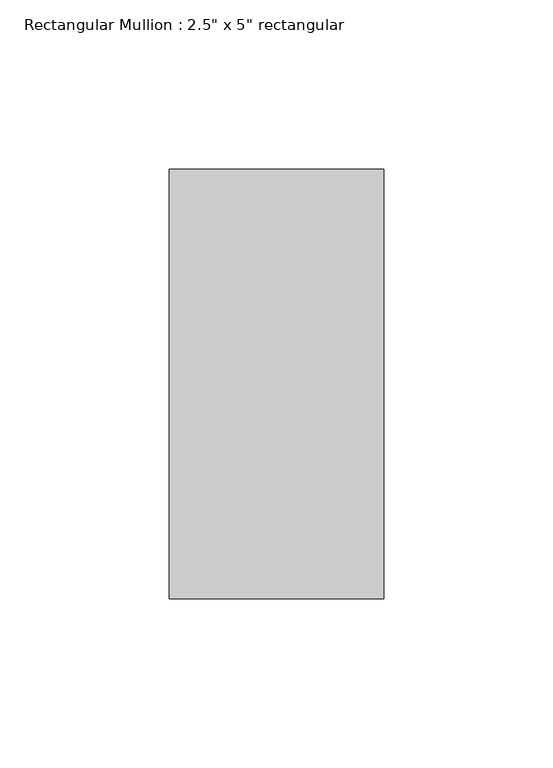
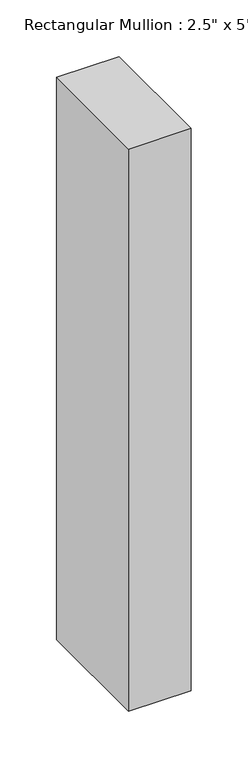
"""IFC4 building model written with IfcOpenShell, lengths in millimetres: member geometry."""

from ifc_helpers import new_model, si_unit, frame, origin, place, context, project, spatial, polyline, outline, extrude, source, transform, mapped, element, save


def member_00d8fd3b(model_context):
    return source(origin(), model_context, "Body", "SweptSolid", [
        extrude(outline(polyline([(0.0, 63.5), (0.0, -63.5), (-63.5, -63.5), (-63.5, 63.5), (0.0, 63.5)])), frame((0.0, 0.0, -604.4408868), z_axis=(0.0, 0.0, 1.0), x_axis=(1.0, 0.0, 0.0)), (0.0, 0.0, 1.0), 604.4408868),
    ])


if __name__ == "__main__":
    model = new_model("IFC4")
    model_context = context("Model", 3, world=origin())
    ifc_project = project(units=[si_unit("LENGTHUNIT", "METRE", prefix="MILLI")], contexts=[model_context])
    site = spatial("IfcSite", under=ifc_project)
    building = spatial("IfcBuilding", under=site)
    placement = place(None, origin())
    member_shape = member_00d8fd3b(model_context)
    element("IfcMember", 1, ObjectType="Rectangular Mullion : 2.5\" x 5\" rectangular", at=placement, inside=building, context=model_context, shape_type="MappedRepresentation", body=[
        mapped(member_shape, transform((0.0, 0.0, 0.0), x_axis=(1.0, 0.0, 0.0), y_axis=(0.0, 1.0, 0.0), z_axis=(0.0, 0.0, 1.0))),
    ])
    save(model, "model.ifc")

# Revit data of these elements
# Type "Rectangular Mullion : 2.5\" x 5\" rectangular"
#   built-in parameter 1007304 = 0.416667 (stored number, unit not read)
#   built-in parameter 1007301 = 0.104167 (stored number, unit not read)
#   built-in parameter 1007300 = 0.104167 (stored number, unit not read)
# Element 1 (IfcMember, "Rectangular Mullion : 2.5\" x 5\" rectangular")
#   Materials on its faces: "Aluminum"
# Materials
#   "Aluminum": class "Metal", colour RGB 247 247 247, transparency 0, Description = "Aluminum 6061", Cost = 0
